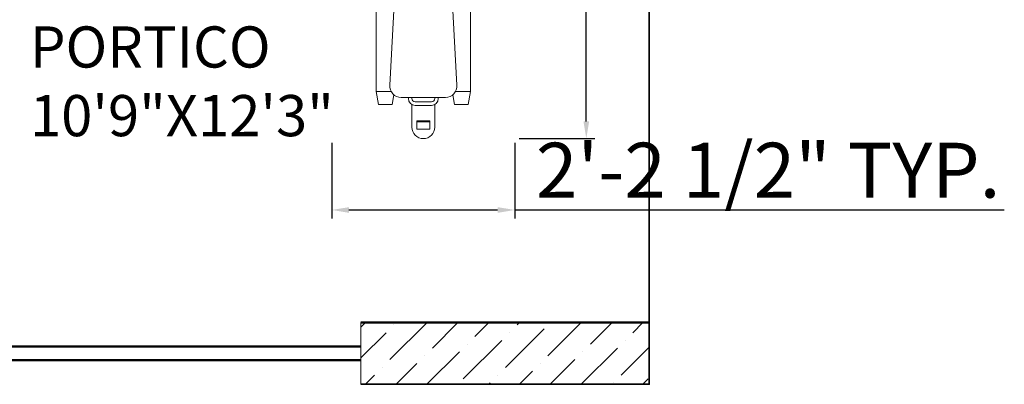
# Model space of a CAD drawing. Units: inches. Extents: x 3354 to 4308, y 1668 to 2317.
# Tile 3 of 11: x 3689 to 3832, y 1754 to 1807. Entities that reach past the tile are written whole.
import ezdxf

# ---------------------------------------------------------------- set-up
doc = ezdxf.new("R2010")
doc.units = ezdxf.units.IN
for name, color, linetype, lineweight in [('A-ANNO-DIMS', 2, 'Continuous', 18), ('A-AREA-IDEN', 3, 'Continuous', 18), ('A-EQPM', 9, 'Continuous', 18), ('A-GLAZ', 4, 'Continuous', 18), ('A-WALL', 7, 'Continuous', 50), ('A-WALL-PATT', 8, 'Continuous', 13), ('C-PROP', 1, 'Continuous', 35)]:
    doc.layers.add(name, color=color, linetype=linetype, lineweight=lineweight)
doc.styles.get("Standard").update_dxf_attribs({"font": 'arial.ttf'})
doc.dimstyles.new('ISO-25', dxfattribs={"dimtxt": 8, "dimasz": 2.5, "dimexe": 1.25, "dimexo": 0.625, "dimtad": 1, "dimdec": 1, "dimlunit": 3, "dimtxsty": 'Standard', "dimcen": 2.5, "dimadec": 0, "dimazin": 0, "dimtfac": 1, "dimtdec": 1, "dimtmove": 0, "dimatfit": 3, "dimfxl": 1, "dimarcsym": 0})

# ---------------------------------------------------------------- blocks, each defined once
blk = doc.blocks.new('BIKE')
for p, q in [((34846.04, 15170.344), (34846.04, 15168.869)), ((34847.863, 15170.344), (34847.863, 15168.869)), ((34845.812, 15167.865), (34845.812, 15160.698)), ((34845.812, 15167.865), (34845.812, 15160.698)), ((34848.09, 15167.865), (34848.09, 15160.698)), ((34844.293, 15164.403), (34844.293, 15160.811)), ((34845.432, 15164.403), (34845.432, 15160.811)), ((34848.47, 15164.403), (34848.47, 15160.811)), ((34849.609, 15164.403), (34849.609, 15160.811)), ((34845.432, 15164.099), (34845.812, 15164.099)), ((34845.432, 15163.85), (34845.812, 15163.85)), ((34848.47, 15164.099), (34848.09, 15164.099)), ((34848.47, 15163.85), (34848.09, 15163.85)), ((34844.407, 15160.811), (34844.407, 15157.429)), ((34845.318, 15160.811), (34845.318, 15157.429)), ((34848.513, 15160.529), (34845.39, 15160.529)), ((34845.39, 15160.235), (34845.39, 15160.529)), ((34845.39, 15160.235), (34845.39, 15160.529)), ((34848.513, 15160.235), (34848.513, 15160.529)), ((34848.584, 15160.811), (34848.584, 15157.429)), ((34849.496, 15160.811), (34849.496, 15157.429)), ((34848.513, 15160.235), (34845.39, 15160.235)), ((34845.318, 15157.919), (34846.037, 15157.919)), ((34848.584, 15157.919), (34847.865, 15157.919)), ((34840.801, 15156.108), (34844.559, 15156.882)), ((34844.293, 15156.871), (34844.293, 15157.169)), ((34844.407, 15156.871), (34844.407, 15156.851)), ((34844.559, 15156.882), (34846.951, 15156.882)), ((34845.432, 15156.871), (34845.432, 15157.169)), ((34849.344, 15156.882), (34846.951, 15156.882)), ((34848.47, 15156.871), (34848.47, 15157.169)), ((34853.102, 15156.108), (34849.344, 15156.882)), ((34849.496, 15156.871), (34849.496, 15156.851)), ((34849.609, 15156.871), (34849.609, 15157.169)), ((34837.837, 15154.891), (34840.367, 15155.929)), ((34840.194, 15156.351), (34840.299, 15156.394)), ((34840.194, 15156.351), (34840.799, 15154.875)), ((34840.299, 15156.394), (34840.905, 15154.919)), ((34840.472, 15155.973), (34840.801, 15156.108)), ((34841.001, 15155.451), (34844.628, 15156.198)), ((34844.855, 15144.722), (34843.012, 15155.865)), ((34844.628, 15156.198), (34846.951, 15156.198)), ((34849.274, 15156.198), (34846.951, 15156.198)), ((34849.048, 15144.722), (34850.89, 15155.865)), ((34852.901, 15155.451), (34849.274, 15156.198)), ((34853.603, 15156.394), (34852.998, 15154.919)), ((34853.43, 15155.973), (34853.102, 15156.108)), ((34853.709, 15156.351), (34853.103, 15154.875)), ((34856.065, 15154.891), (34853.536, 15155.929)), ((34853.709, 15156.351), (34853.603, 15156.394)), ((34837.837, 15154.891), (34838.097, 15154.259)), ((34838.097, 15154.259), (34840.626, 15155.297)), ((34840.732, 15155.34), (34841.001, 15155.451)), ((34840.799, 15154.875), (34840.905, 15154.919)), ((34843.061, 15154.2), (34843.225, 15154.581)), ((34850.842, 15154.2), (34850.678, 15154.581)), ((34853.171, 15155.34), (34852.901, 15155.451)), ((34853.103, 15154.875), (34852.998, 15154.919)), ((34855.805, 15154.259), (34853.276, 15155.297)), ((34856.065, 15154.891), (34855.805, 15154.259)), ((34842.804, 15152.592), (34843.061, 15154.2)), ((34851.099, 15152.592), (34850.842, 15154.2)), ((34843.328, 15151.093), (34843.52, 15152.795)), ((34850.574, 15151.093), (34850.383, 15152.795)), ((34842.703, 15150.307), (34842.804, 15152.592)), ((34851.199, 15150.307), (34851.099, 15152.592)), ((34843.23, 15147.751), (34843.328, 15151.093)), ((34850.673, 15147.751), (34850.574, 15151.093)), ((34840.971, 15150.307), (34843.305, 15150.307)), ((34840.971, 15149.813), (34840.971, 15150.307)), ((34843.29, 15149.813), (34840.971, 15149.813)), ((34842.703, 15144.873), (34842.703, 15149.813)), ((34852.932, 15150.307), (34850.598, 15150.307)), ((34850.612, 15149.813), (34852.932, 15149.813)), ((34851.199, 15144.873), (34851.199, 15149.813)), ((34852.932, 15149.813), (34852.932, 15150.307)), ((34843.23, 15144.145), (34843.23, 15147.751)), ((34850.673, 15144.145), (34850.673, 15147.751)), ((34842.703, 15144.873), (34842.248, 15142.195)), ((34842.703, 15144.873), (34843.23, 15144.873)), ((34851.199, 15144.873), (34850.673, 15144.873)), ((34851.199, 15144.873), (34851.655, 15142.195)), ((34847.846, 15144.636), (34846.057, 15144.636)), ((34844.464, 15143.561), (34843.601, 15128.195)), ((34843.854, 15143.464), (34844.07, 15142.195)), ((34843.913, 15143.462), (34844.458, 15143.462)), ((34849.439, 15143.561), (34850.301, 15128.195)), ((34849.989, 15143.462), (34849.444, 15143.462)), ((34850.048, 15143.464), (34849.832, 15142.195)), ((34842.248, 15142.195), (34844.07, 15142.195)), ((34842.248, 15137.821), (34842.248, 15142.195)), ((34844.07, 15137.821), (34844.07, 15142.195)), ((34851.655, 15142.195), (34849.832, 15142.195)), ((34849.832, 15137.821), (34849.832, 15142.195)), ((34851.655, 15137.821), (34851.655, 15142.195)), ((34841.794, 15137.821), (34844.142, 15137.821)), ((34841.794, 15137.328), (34841.794, 15137.821)), ((34844.114, 15137.328), (34841.794, 15137.328)), ((34842.248, 15127.566), (34842.248, 15137.328)), ((34844.07, 15136.554), (34844.07, 15137.328)), ((34852.108, 15137.821), (34849.761, 15137.821)), ((34849.789, 15137.328), (34852.108, 15137.328)), ((34849.832, 15136.554), (34849.832, 15137.328)), ((34851.655, 15127.566), (34851.655, 15137.328)), ((34852.108, 15137.328), (34852.108, 15137.821)), ((34842.248, 15127.566), (34843.75, 15127.566)), ((34842.248, 15127.566), (34842.476, 15126.269)), ((34844.015, 15127.251), (34843.843, 15126.269)), ((34849.887, 15127.251), (34850.06, 15126.269)), ((34851.655, 15127.566), (34850.153, 15127.566)), ((34851.655, 15127.566), (34851.427, 15126.269)), ((34842.476, 15126.269), (34843.843, 15126.269)), ((34849.164, 15126.992), (34844.739, 15126.992)), ((34845.47, 15126.992), (34845.47, 15126.882)), ((34845.812, 15126.992), (34845.812, 15126.882)), ((34845.812, 15126.29), (34845.812, 15124.029)), ((34847.749, 15126.54), (34846.154, 15126.54)), ((34847.749, 15126.198), (34846.154, 15126.198)), ((34848.09, 15126.992), (34848.09, 15126.882)), ((34848.09, 15126.29), (34848.09, 15124.029)), ((34848.432, 15126.992), (34848.432, 15126.882)), ((34851.427, 15126.269), (34850.06, 15126.269)), ((34846.291, 15123.822), (34846.291, 15124.661)), ((34846.291, 15124.661), (34847.611, 15124.661)), ((34846.291, 15124.547), (34847.611, 15124.547)), ((34847.611, 15124.661), (34847.611, 15123.822)), ((34847.611, 15123.822), (34846.291, 15123.822))]:
    blk.add_line(p, q)
for points in [[(34845.812, 15167.865, -0.068977), (34845.904, 15168.528, -0.081012), (34846.146, 15169.045, -0.107014), (34846.54, 15169.419, -0.137239), (34846.951, 15169.534, -0.137239), (34847.362, 15169.419, -0.107014), (34847.757, 15169.045, -0.081012), (34847.999, 15168.528, -0.068977), (34848.09, 15167.865, -0.068977)], [(34845.432, 15164.403, 0.125099), (34845.392, 15164.563, 0.105827), (34845.265, 15164.71, 0.086577), (34845.087, 15164.802, 0.0766), (34844.863, 15164.837, 0.0766), (34844.638, 15164.802, 0.086577), (34844.46, 15164.71, 0.105827), (34844.334, 15164.563, 0.125099), (34844.293, 15164.403, 0.125099)], [(34848.47, 15164.403, -0.125099), (34848.511, 15164.563, -0.105827), (34848.637, 15164.71, -0.086577), (34848.816, 15164.802, -0.0766), (34849.04, 15164.837, -0.0766), (34849.264, 15164.802, -0.086577), (34849.443, 15164.71, -0.105827), (34849.569, 15164.563, -0.125099), (34849.609, 15164.403, -0.125099)], [(34845.318, 15160.551, 0.067261), (34845.392, 15160.652, 0.125099), (34845.432, 15160.811, 0.125099), (34845.392, 15160.971, 0.105827), (34845.265, 15161.118, 0.086577), (34845.087, 15161.211, 0.0766), (34844.863, 15161.245, 0.0766), (34844.638, 15161.211, 0.086577), (34844.46, 15161.118, 0.105827), (34844.334, 15160.971, 0.125099), (34844.293, 15160.811, 0.125099)], [(34844.293, 15160.811, 0.125099), (34844.334, 15160.652, 0.067261), (34844.407, 15160.551, 0.086577)], [(34845.318, 15160.811, 0.125099), (34845.292, 15160.917, 0.105827), (34845.196, 15161.028, 0.086577), (34845.053, 15161.102, 0.0766), (34844.863, 15161.132, 0.0766), (34844.673, 15161.102, 0.086577), (34844.529, 15161.028, 0.105827), (34844.434, 15160.917, 0.125099), (34844.407, 15160.811, 0.125099)], [(34848.584, 15160.551, -0.067261), (34848.511, 15160.652, -0.125099), (34848.47, 15160.811, -0.125099), (34848.511, 15160.971, -0.105827), (34848.637, 15161.118, -0.086577), (34848.816, 15161.211, -0.0766), (34849.04, 15161.245, -0.0766), (34849.264, 15161.211, -0.086577), (34849.443, 15161.118, -0.105827), (34849.569, 15160.971, -0.125099), (34849.609, 15160.811, -0.125099)], [(34848.584, 15160.811, -0.125099), (34848.611, 15160.917, -0.105827), (34848.706, 15161.028, -0.086577), (34848.85, 15161.102, -0.0766), (34849.04, 15161.132, -0.0766), (34849.23, 15161.102, -0.086577), (34849.374, 15161.028, -0.105827), (34849.469, 15160.917, -0.125099), (34849.496, 15160.811, -0.125099)], [(34849.609, 15160.811, -0.125099), (34849.569, 15160.652, -0.067261), (34849.496, 15160.551, -0.086577)], [(34846.951, 15157.368, -0.163989), (34846.412, 15157.55, -0.105862), (34845.847, 15158.208, -0.069323), (34845.519, 15159.08, -0.055531), (34845.39, 15160.235, -0.055531)], [(34848.513, 15160.235, -0.055531), (34848.384, 15159.08, -0.069323), (34848.055, 15158.208, -0.105862), (34847.49, 15157.55, -0.163989), (34846.951, 15157.368, -0.163989)], [(34845.432, 15157.169, 0.125099), (34845.392, 15157.329, 0.105827), (34845.265, 15157.476, 0.086577), (34845.087, 15157.568, 0.0766), (34844.863, 15157.603, 0.0766), (34844.638, 15157.568, 0.086577), (34844.46, 15157.476, 0.105827), (34844.334, 15157.329, 0.125099), (34844.293, 15157.169, 0.125099)], [(34848.47, 15157.169, -0.125099), (34848.511, 15157.329, -0.105827), (34848.637, 15157.476, -0.086577), (34848.816, 15157.568, -0.0766), (34849.04, 15157.603, -0.0766), (34849.264, 15157.568, -0.086577), (34849.443, 15157.476, -0.105827), (34849.569, 15157.329, -0.125099), (34849.609, 15157.169, -0.125099)], [(34845.432, 15156.882, 0.117252), (34845.392, 15157.031, 0.105827), (34845.265, 15157.178, 0.086577), (34845.087, 15157.271, 0.0766), (34844.863, 15157.306, 0.0766), (34844.638, 15157.271, 0.086577), (34844.46, 15157.178, 0.105827), (34844.334, 15157.031, 0.125099), (34844.293, 15156.871, 0.125099)], [(34844.293, 15156.871, 0.032819), (34844.296, 15156.828, 0.067261)], [(34845.318, 15156.882, 0.113202), (34845.292, 15156.977, 0.105827), (34845.196, 15157.088, 0.086577), (34845.053, 15157.162, 0.0766), (34844.863, 15157.192, 0.0766), (34844.673, 15157.162, 0.086577), (34844.529, 15157.088, 0.105827), (34844.434, 15156.977, 0.125099), (34844.407, 15156.871, 0.125099)], [(34848.47, 15156.882, -0.117252), (34848.511, 15157.031, -0.105827), (34848.637, 15157.178, -0.086577), (34848.816, 15157.271, -0.0766), (34849.04, 15157.306, -0.0766), (34849.264, 15157.271, -0.086577), (34849.443, 15157.178, -0.105827), (34849.569, 15157.031, -0.125099), (34849.609, 15156.871, -0.125099)], [(34848.584, 15156.882, -0.113202), (34848.611, 15156.977, -0.105827), (34848.706, 15157.088, -0.086577), (34848.85, 15157.162, -0.0766), (34849.04, 15157.192, -0.0766), (34849.23, 15157.162, -0.086577), (34849.374, 15157.088, -0.105827), (34849.469, 15156.977, -0.125099), (34849.496, 15156.871, -0.125099)], [(34849.609, 15156.871, -0.032819), (34849.607, 15156.828, -0.067261)]]:
    blk.add_lwpolyline(points, format="xyb")
for centre, radius, start, end in [((34846.951, 15157.242), 3.638, 64.58823, 115.41177), ((34844.552, 15156.324), 1.595, 95.22072, 171.67796), ((34849.35, 15156.324), 1.595, 8.32204, 84.77928), ((34843.861, 15154.923), 0.684, 90, 189.38978), ((34846.951, 15140.123), 15.789, 78.71287, 101.28713), ((34850.042, 15154.923), 0.684, 350.61022, 90), ((34843.913, 15144.145), 0.684, 180, 270), ((34846.003, 15142.998), 1.639, 88.11253, 159.92642), ((34845.529, 15144.833), 0.684, 189.38978, 226.48769), ((34847.9, 15142.998), 1.639, 20.07358, 91.88747), ((34848.373, 15144.833), 0.684, 313.51231, 350.61022), ((34849.989, 15144.145), 0.684, 270, 0), ((34844.739, 15128.131), 1.139, 176.78649, 270), ((34849.164, 15128.131), 1.139, 270, 3.21351), ((34846.154, 15126.882), 0.684, 180, 270), ((34846.154, 15126.882), 0.342, 180, 270), ((34847.749, 15126.882), 0.684, 270, 0), ((34847.749, 15126.882), 0.342, 270, 0), ((34846.951, 15124.029), 1.139, 180, 0)]:
    blk.add_arc(centre, radius, start, end)
blk = doc.blocks.new('*D70')
at = {"layer": 'A-ANNO-DIMS', "color": 0, "lineweight": -2, "transparency": 16777216}
for p, q in [((3771.12, 1859.52), (3771.12, 2000.47)), ((3761.34, 1859.52), (3772.37, 1859.52)), ((3771.12, 1792.61), (3771.12, 1857.02)), ((3761.34, 1790.11), (3772.37, 1790.11))]:
    blk.add_line(p, q, dxfattribs=at)
at = {"layer": 'A-ANNO-DIMS', "color": 0, "transparency": 16777216}
for points in [[(3770.71, 1857.02), (3771.54, 1857.02), (3771.12, 1859.52)], [(3770.71, 1792.61), (3771.54, 1792.61), (3771.12, 1790.11)]]:
    blk.add_solid(points, dxfattribs=at)
at = {"layer": 'Defpoints', "color": 0, "transparency": 16777216}
for p in [(3760.71, 1859.52), (3771.12, 1859.52), (3760.71, 1790.11)]:
    blk.add_point(p, dxfattribs=at)
at = {"layer": 'A-ANNO-DIMS', "color": 0, "transparency": 16777216, "insert": (3766.36, 1931.24), "char_height": 8, "attachment_point": 5, "rotation": 90}
blk.add_mtext('MOTORBIKE 5\'-9 1/2" TYP.', dxfattribs=at)
blk = doc.blocks.new('*D71')
at = {"layer": 'A-ANNO-DIMS', "color": 0, "lineweight": -2, "transparency": 16777216}
for p, q in [((3734.05, 1789.48), (3734.05, 1778.45)), ((3760.71, 1789.48), (3760.71, 1778.45)), ((3736.55, 1779.7), (3758.21, 1779.7)), ((3760.71, 1779.7), (3832, 1779.7))]:
    blk.add_line(p, q, dxfattribs=at)
at = {"layer": 'A-ANNO-DIMS', "color": 0, "transparency": 16777216}
for points in [[(3736.55, 1780.11), (3736.55, 1779.28), (3734.05, 1779.7)], [(3758.21, 1780.11), (3758.21, 1779.28), (3760.71, 1779.7)]]:
    blk.add_solid(points, dxfattribs=at)
at = {"layer": 'Defpoints', "color": 0, "transparency": 16777216}
for p in [(3734.05, 1790.11), (3760.71, 1790.11), (3760.71, 1779.7)]:
    blk.add_point(p, dxfattribs=at)
at = {"layer": 'A-ANNO-DIMS', "color": 0, "transparency": 16777216, "insert": (3797.61, 1784.46), "char_height": 8, "attachment_point": 5}
blk.add_mtext('2\'-2 1/2" TYP.', dxfattribs=at)

msp = doc.modelspace()

# ---------------------------------------------------------------- hatches: boundary and pattern name
at = {"layer": 'A-WALL-PATT', "transparency": 33554687}
h = msp.add_hatch(dxfattribs=at)
h.set_pattern_fill('ANSI36', color=256)
h.paths.add_polyline_path([(3666.28, 1763.3), (3636.28, 1763.3), (3636.28, 1754.3), (3666.28, 1754.3)])
h.paths.add_polyline_path([(3780.28, 1763.3), (3738.28, 1763.3), (3738.28, 1754.3), (3780.28, 1754.3)])

# ---------------------------------------------------------------- linework, layer by layer
at = {"layer": 'A-GLAZ'}
msp.add_line((3738.28, 1763.3), (3738.28, 1754.3), dxfattribs=at)
at = {"layer": 'A-WALL'}
for p, q in [((3738.28, 1763.3), (3780.28, 1763.3)), ((3666.28, 1759.8), (3738.28, 1759.8)), ((3666.28, 1757.8), (3738.28, 1757.8))]:
    msp.add_line(p, q, dxfattribs=at)
at = {"layer": 'C-PROP'}
msp.add_lwpolyline([(3738.28, 1754.3), (3780.28, 1754.3), (3780.28, 2294.3), (3396.28, 2294.3), (3396.28, 1754.3), (3576.28, 1754.3)], dxfattribs=at)

# ---------------------------------------------------------------- block references
at = {"layer": 'A-EQPM', "xscale": 1.462635365130814, "yscale": 1.462635365130814, "zscale": 1.462635365130814}
msp.add_blockref('BIKE', (-47221, -20329.17), dxfattribs=at)

# ---------------------------------------------------------------- texts
at = {"layer": 'A-AREA-IDEN', "insert": (3690.09, 1806.45), "char_height": 6, "attachment_point": 1}
msp.add_mtext_dynamic_manual_height_columns('PORTICO\\P10\'9"X12\'3"', width=74.5832, gutter_width=12.5, heights=[0], dxfattribs=at)

# ---------------------------------------------------------------- dimensions: what is measured, and where the dimension line sits
at = {"layer": 'A-ANNO-DIMS'}
dim = msp.add_linear_dim(base=(3771.12, 1859.52), p1=(3760.71, 1790.11), p2=(3760.71, 1859.52), angle=90, text='MOTORBIKE <> TYP.', dimstyle='ISO-25', override={"dimdec": 1, "dimrnd": 0, "dimzin": 1, "dimlunit": 4, "dimfrac": 2}, dxfattribs=at)
dim.commit()
dim.dimension.update_dxf_attribs({"geometry": '*D70', "text_midpoint": (3766.36, 1931.24)})
dim = msp.add_linear_dim(base=(3760.71, 1779.7), p1=(3734.05, 1790.11), p2=(3760.71, 1790.11), text='<> TYP.', dimstyle='ISO-25', override={"dimdec": 1, "dimrnd": 0, "dimzin": 1, "dimlunit": 4, "dimfrac": 2}, dxfattribs=at)
dim.commit()
dim.dimension.update_dxf_attribs({"geometry": '*D71', "text_midpoint": (3797.61, 1784.46)})

doc.saveas('drawing.dxf')
